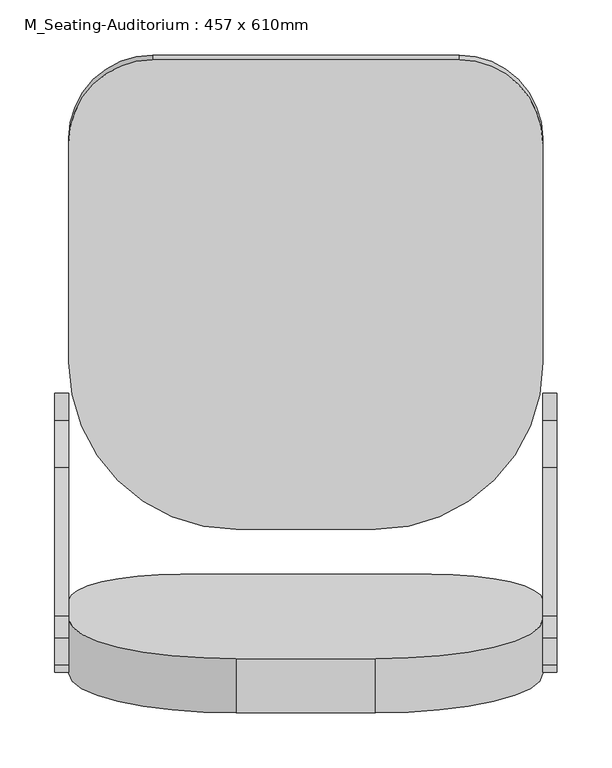
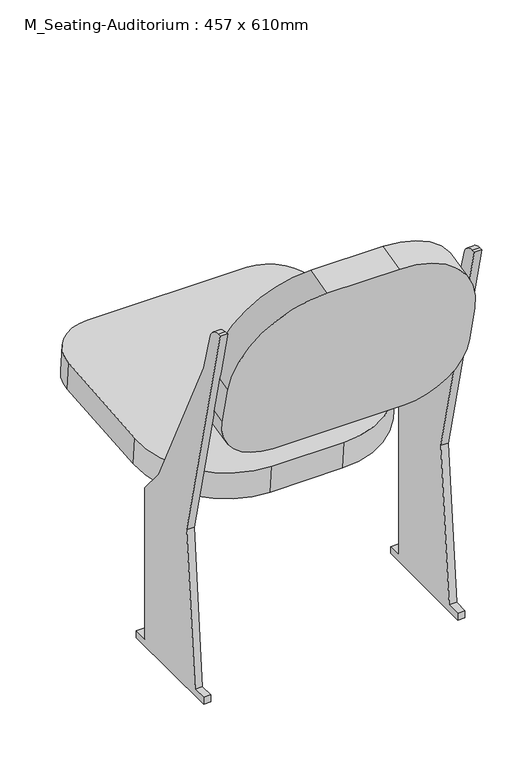
"""IFC4 building model written with IfcOpenShell, lengths in millimetres: furniture geometry, M_Seating-Auditorium : 457 x 610mm."""

from ifc_helpers import new_model, si_unit, point, frame, frame_2d, origin, place, context, project, spatial, polyline, circle_curve, trimmed, segment, composite_curve, outline, extrude, source, transform, mapped, element, save


def m_seating_auditorium_457_x_610mm_3d1d9cbc(model_context):
    return source(origin(), model_context, "Body", "SweptSolid", [
        extrude(outline(composite_curve([segment(polyline([(0.0, 0.0), (127.0, 0.0)]), True, "CONTINUOUS"), segment(trimmed(circle_curve(frame_2d((127.0, -152.4)), 152.4), [point((127.0, 0.0))], [point((279.4, -152.4))], False, "CARTESIAN"), True, "CONTINUOUS"), segment(polyline([(279.4, -152.4), (279.4, -224.0588601)]), True, "CONTINUOUS"), segment(trimmed(circle_curve(frame_2d((177.8, -224.0588601)), 101.6), [point((279.4, -224.0588601))], [point((177.8, -325.6588601))], False, "CARTESIAN"), True, "CONTINUOUS"), segment(polyline([(177.8, -325.6588601), (-50.8, -325.6588601)]), True, "CONTINUOUS"), segment(trimmed(circle_curve(frame_2d((-50.8, -224.0588601)), 101.6), [point((-50.8, -325.6588601))], [point((-152.4, -224.0588601))], False, "CARTESIAN"), True, "CONTINUOUS"), segment(polyline([(-152.4, -224.0588601), (-152.4, -152.4)]), True, "CONTINUOUS"), segment(trimmed(circle_curve(frame_2d((0.0, -152.4)), 152.4), [point((-152.4, -152.4))], [point((0.0, 0.0))], False, "CARTESIAN"), True, "CONTINUOUS")], self_intersect=False)), frame((224.2278689, -101.3396919, 755.9484479), z_axis=(0.0, 0.9717404775047361, 0.23605178325712217), x_axis=(-1.0, 0.0, 0.0)), (0.0, 0.0, 1.0), 50.8),
        extrude(outline(composite_curve([segment(trimmed(circle_curve(frame_2d((0.0, -76.2)), 76.2), [point((0.0, 0.0))], [point((76.2, -76.2))], False, "CARTESIAN"), True, "CONTINUOUS"), segment(polyline([(76.2, -76.2), (76.2, -276.4123505)]), True, "CONTINUOUS"), segment(trimmed(circle_curve(frame_2d((-76.2, -276.4123505)), 152.4), [point((76.2, -276.4123505))], [point((-76.2, -428.8123506))], False, "CARTESIAN"), True, "CONTINUOUS"), segment(polyline([(-76.2, -428.8123506), (-203.2, -428.8123506)]), True, "CONTINUOUS"), segment(trimmed(circle_curve(frame_2d((-203.2, -276.4123505)), 152.4), [point((-203.2, -428.8123506))], [point((-355.6, -276.4123505))], False, "CARTESIAN"), True, "CONTINUOUS"), segment(polyline([(-355.6, -276.4123505), (-355.6, -76.2)]), True, "CONTINUOUS"), segment(trimmed(circle_curve(frame_2d((-279.4, -76.2)), 76.2), [point((-355.6, -76.2))], [point((-279.4, 0.0))], False, "CARTESIAN"), True, "CONTINUOUS"), segment(polyline([(-279.4, 0.0), (0.0, 0.0)]), True, "CONTINUOUS")], self_intersect=False)), frame((300.4278689, 497.5245173, 321.2380213), z_axis=(0.0, -0.08715574274765496, 0.9961946980917459), x_axis=(1.0, 0.0, 0.0)), (0.0, 0.0, 1.0), 50.8),
        extrude(outline(composite_curve([segment(polyline([(-13.3245902, 0.0), (-13.3245902, 12.7), (12.0754098, 12.7), (37.4754098, 292.1), (-64.1245902, 711.2), (-57.883846, 711.2)]), True, "CONTINUOUS"), segment(trimmed(circle_curve(frame_2d((-57.883846, 685.8)), 25.4), [point((-57.883846, 711.2))], [point((-33.4611378, 692.7779166))], False, "CARTESIAN"), True, "CONTINUOUS"), segment(polyline([(-33.4611378, 692.7779166), (-13.3245902, 622.3), (121.8491486, 342.9), (164.4754098, 292.1), (164.4754098, 12.7), (189.8754098, 12.7), (189.8754098, 0.0), (-13.3245902, 0.0)]), True, "CONTINUOUS")], self_intersect=False)), frame((-67.8721311, 0.0, 0.0), z_axis=(1.0, 0.0, 0.0), x_axis=(0.0, 1.0, 0.0)), (0.0, 0.0, 1.0), 12.7),
        extrude(outline(composite_curve([segment(polyline([(-13.3245902, 12.7), (12.0754098, 12.7), (37.4754098, 292.1), (-64.1245902, 711.2), (-57.883846, 711.2)]), True, "CONTINUOUS"), segment(trimmed(circle_curve(frame_2d((-57.883846, 685.8)), 25.4), [point((-57.883846, 711.2))], [point((-33.4611378, 692.7779166))], False, "CARTESIAN"), True, "CONTINUOUS"), segment(polyline([(-33.4611378, 692.7779166), (-13.3245902, 622.3), (121.8491486, 342.9), (164.4754098, 292.1), (164.4754098, 12.7), (189.8754098, 12.7), (189.8754098, 0.0), (-13.3245902, 0.0), (-13.3245902, 12.7)]), True, "CONTINUOUS")], self_intersect=False)), frame((376.6278689, 0.0, 0.0), z_axis=(1.0, 0.0, 0.0), x_axis=(0.0, 1.0, 0.0)), (0.0, 0.0, 1.0), 12.7),
    ])


if __name__ == "__main__":
    model = new_model("IFC4")
    model_context = context("Model", 3, world=origin())
    ifc_project = project(units=[si_unit("LENGTHUNIT", "METRE", prefix="MILLI")], contexts=[model_context])
    site = spatial("IfcSite", under=ifc_project)
    building = spatial("IfcBuilding", under=site)
    placement = place(None, origin())
    m_seating_auditorium_457_x_610mm_shape = m_seating_auditorium_457_x_610mm_3d1d9cbc(model_context)
    element("IfcFurniture", 1, ObjectType="M_Seating-Auditorium : 457 x 610mm", at=placement, inside=building, context=model_context, shape_type="MappedRepresentation", body=[
        mapped(m_seating_auditorium_457_x_610mm_shape, transform((0.0, 0.0, 0.0), x_axis=(1.0, 0.0, 0.0), y_axis=(0.0, 1.0, 0.0), z_axis=(0.0, 0.0, 1.0))),
    ])
    save(model, "model.ifc")

# Revit data of these elements
# Type "M_Seating-Auditorium : 457 x 610mm"
#   Seat/Back Material = Linen, Beige
#   Frame Material = Steel, Paint Finish, Dark Gray, Matte
#   Default Elevation = 0
# Element 1 (IfcFurniture, "M_Seating-Auditorium : 457 x 610mm")
#   Materials on its faces: "Steel, Paint Finish, Dark Gray, Matte", "Linen, Beige"
# Materials
#   "Linen, Beige": class "Textile", colour RGB 249 239 230, transparency 0, Description = "Linen, beige", Cost = 0
#   "Steel, Paint Finish, Dark Gray, Matte": class "Metal", colour RGB 0 0 0, transparency 0, Description = "Steel, paint finish, dark gray, matte", Cost = 0
